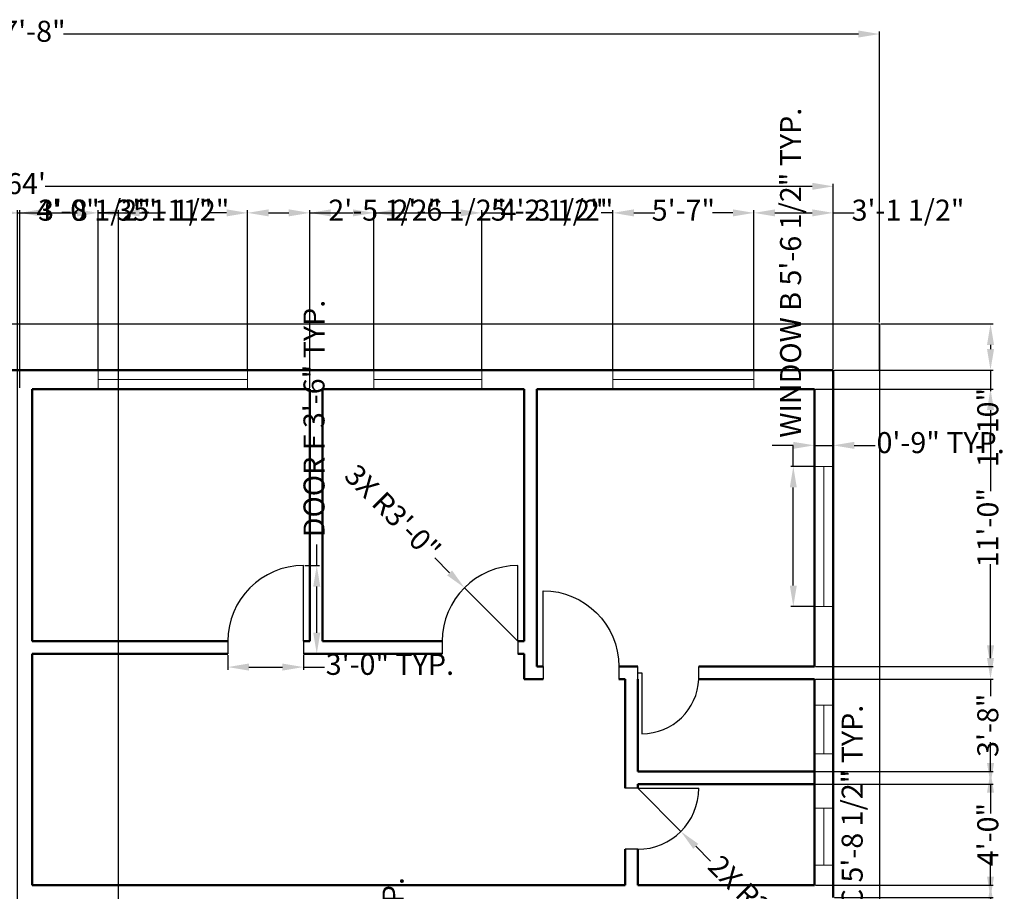
# Model space of a CAD drawing. Units: inches. Extents: x 3237 to 4201, y 2949 to 4053.
# Tile 5 of 5: x 3725 to 4193, y 3638 to 4053. Entities that reach past the tile are written whole.
import ezdxf

# ---------------------------------------------------------------- set-up
doc = ezdxf.new("R2010")
doc.units = ezdxf.units.IN
for name, color, linetype, lineweight in [('A-ANNO-DIMS', 2, 'Continuous', 18), ('A-DOOR', 3, 'Continuous', 25), ('A-GLAZ', 4, 'Continuous', 18), ('A-WALL', 7, 'Continuous', 50), ('C-PROP', 6, 'Continuous', 25)]:
    doc.layers.add(name, color=color, linetype=linetype, lineweight=lineweight)
doc.styles.get("Standard").update_dxf_attribs({"font": 'arial.ttf'})
doc.dimstyles.new('ISO-25', dxfattribs={"dimtxt": 10, "dimasz": 10, "dimexe": 1.25, "dimexo": 0.625, "dimtad": 0, "dimdec": 0, "dimlunit": 3, "dimtxsty": 'Standard', "dimcen": 2.5, "dimadec": 0, "dimazin": 0, "dimtfac": 1, "dimtdec": 0, "dimtmove": 0, "dimatfit": 3, "dimfxl": 1, "dimarcsym": 0})

# ---------------------------------------------------------------- blocks, each defined once
blk = doc.blocks.new('*D1')
at = {"layer": 'A-ANNO-DIMS', "color": 0, "lineweight": -2, "transparency": 16777216}
for p, q in [((3321.52, 3908.6), (3321.52, 4047.14)), ((4133.52, 3908.6), (4133.52, 4047.14)), ((3331.52, 4045.89), (3709.69, 4045.89)), ((4123.52, 4045.89), (3745.35, 4045.89))]:
    blk.add_line(p, q, dxfattribs=at)
at = {"layer": 'A-ANNO-DIMS', "color": 0, "transparency": 16777216}
for points in [[(3331.52, 4047.56), (3331.52, 4044.22), (3321.52, 4045.89)], [(4123.52, 4047.56), (4123.52, 4044.22), (4133.52, 4045.89)]]:
    blk.add_solid(points, dxfattribs=at)
at = {"layer": 'Defpoints', "color": 0, "transparency": 16777216}
for p in [(4133.52, 4045.89), (3321.52, 3907.98), (4133.52, 3907.98)]:
    blk.add_point(p, dxfattribs=at)
at = {"layer": 'A-ANNO-DIMS', "color": 0, "transparency": 16777216, "insert": (3727.52, 4045.89), "char_height": 10, "attachment_point": 5}
blk.add_mtext('67\'-8"', dxfattribs=at)
blk = doc.blocks.new('*D3')
at = {"layer": 'A-ANNO-DIMS', "color": 0, "lineweight": -2, "transparency": 16777216}
for p, q in [((3343.52, 3886.6), (3343.52, 3974.66)), ((3353.52, 3973.41), (3718.38, 3973.41)), ((4101.52, 3973.41), (3736.66, 3973.41)), ((4111.52, 3886.6), (4111.52, 3974.66))]:
    blk.add_line(p, q, dxfattribs=at)
at = {"layer": 'A-ANNO-DIMS', "color": 0, "transparency": 16777216}
for points in [[(3353.52, 3975.08), (3353.52, 3971.74), (3343.52, 3973.41)], [(4101.52, 3975.08), (4101.52, 3971.74), (4111.52, 3973.41)]]:
    blk.add_solid(points, dxfattribs=at)
at = {"layer": 'Defpoints', "color": 0, "transparency": 16777216}
for p in [(4111.52, 3973.41), (3343.52, 3885.98), (4111.52, 3885.98)]:
    blk.add_point(p, dxfattribs=at)
at = {"layer": 'A-ANNO-DIMS', "color": 0, "transparency": 16777216, "insert": (3727.52, 3973.41), "char_height": 10, "attachment_point": 5}
blk.add_mtext("64'", dxfattribs=at)
blk = doc.blocks.new('DOOR-29-OFFSET-A')
for p, q in [((0, 26), (0, 32)), ((0, 29), (2, 29)), ((2, 29), (2, 0)), ((29, 26), (29, 32))]:
    blk.add_line(p, q)
blk.add_arc((2, 27.02), 27.02, 270, 357.8382)
blk = doc.blocks.new('DOOR-36')
for p, q in [((36, 6), (36, 42)), ((0, 6), (0, 0)), ((36, 6), (36, 0))]:
    blk.add_line(p, q)
blk.add_arc((36, 6), 36, 90, 180)
blk = doc.blocks.new('DOOR-29')
for p, q in [((6, 29), (0, 29)), ((6, 29), (35, 29)), ((6, 0), (0, 0))]:
    blk.add_line(p, q)
blk.add_arc((6, 29), 29, 270, 0)
blk = doc.blocks.new('WIN-66p71IN')
for p, q in [((0, 66.71), (9, 66.71)), ((4.5, 0), (4.5, 66.71)), ((0, 0), (9, 0))]:
    blk.add_line(p, q)
blk = doc.blocks.new('*D23')
at = {"layer": 'A-ANNO-DIMS', "color": 0, "lineweight": -2, "transparency": 16777216}
for p, q in [((3903.41, 3494.25), (3903.41, 3504.25)), ((3898.15, 3494.25), (3904.66, 3494.25)), ((3903.41, 3464.98), (3903.41, 3484.25)), ((3898.15, 3454.98), (3904.66, 3454.98))]:
    blk.add_line(p, q, dxfattribs=at)
at = {"layer": 'A-ANNO-DIMS', "color": 0, "transparency": 16777216}
for points in [[(3901.75, 3484.25), (3905.08, 3484.25), (3903.41, 3494.25)], [(3901.75, 3464.98), (3905.08, 3464.98), (3903.41, 3454.98)]]:
    blk.add_solid(points, dxfattribs=at)
at = {"layer": 'Defpoints', "color": 0, "transparency": 16777216}
for p in [(3897.52, 3494.25), (3903.41, 3494.25), (3897.52, 3454.98)]:
    blk.add_point(p, dxfattribs=at)
at = {"layer": 'A-ANNO-DIMS', "color": 0, "transparency": 16777216, "insert": (3903.41, 3576.25), "char_height": 10, "attachment_point": 5, "rotation": 90}
blk.add_mtext('DOOR E 3\'-3 1/2" TYP.', dxfattribs=at)
blk = doc.blocks.new('*D25')
at = {"layer": 'A-ANNO-DIMS', "color": 0, "lineweight": -2, "transparency": 16777216}
for p, q in [((3865.82, 3792.98), (3865.82, 3802.98)), ((3860.15, 3792.98), (3867.07, 3792.98)), ((3865.82, 3760.98), (3865.82, 3782.98)), ((3860.15, 3750.98), (3867.07, 3750.98))]:
    blk.add_line(p, q, dxfattribs=at)
at = {"layer": 'A-ANNO-DIMS', "color": 0, "transparency": 16777216}
for points in [[(3864.16, 3782.98), (3867.49, 3782.98), (3865.82, 3792.98)], [(3864.16, 3760.98), (3867.49, 3760.98), (3865.82, 3750.98)]]:
    blk.add_solid(points, dxfattribs=at)
at = {"layer": 'Defpoints', "color": 0, "transparency": 16777216}
for p in [(3859.52, 3792.98), (3865.82, 3792.98), (3859.52, 3750.98)]:
    blk.add_point(p, dxfattribs=at)
at = {"layer": 'A-ANNO-DIMS', "color": 0, "transparency": 16777216, "insert": (3865.82, 3862.94), "char_height": 10, "attachment_point": 5, "rotation": 90}
blk.add_mtext('DOOR F 3\'-6" TYP.', dxfattribs=at)
blk = doc.blocks.new('*D26')
at = {"layer": 'A-ANNO-DIMS', "color": 0, "lineweight": -2, "transparency": 16777216}
for p, q in [((3823.52, 3750.35), (3823.52, 3743.43)), ((3859.52, 3750.35), (3859.52, 3743.43)), ((3833.52, 3744.68), (3849.52, 3744.68)), ((3859.52, 3744.68), (3869.52, 3744.68))]:
    blk.add_line(p, q, dxfattribs=at)
at = {"layer": 'A-ANNO-DIMS', "color": 0, "transparency": 16777216}
for points in [[(3833.52, 3746.35), (3833.52, 3743.01), (3823.52, 3744.68)], [(3849.52, 3746.35), (3849.52, 3743.01), (3859.52, 3744.68)]]:
    blk.add_solid(points, dxfattribs=at)
at = {"layer": 'Defpoints', "color": 0, "transparency": 16777216}
for p in [(3823.52, 3750.98), (3859.52, 3750.98), (3859.52, 3744.68)]:
    blk.add_point(p, dxfattribs=at)
at = {"layer": 'A-ANNO-DIMS', "color": 0, "transparency": 16777216, "insert": (3900.62, 3744.68), "char_height": 10, "attachment_point": 5}
blk.add_mtext('3\'-0" TYP.', dxfattribs=at)
blk = doc.blocks.new('*D29')
at = {"layer": 'A-ANNO-DIMS', "color": 0, "lineweight": -2, "transparency": 16777216}
for p, q in [((4092.52, 3840.16), (4092.52, 3850.16)), ((4101.9, 3840.16), (4091.27, 3840.16)), ((4092.52, 3783.45), (4092.52, 3830.16)), ((4101.9, 3773.45), (4091.27, 3773.45))]:
    blk.add_line(p, q, dxfattribs=at)
at = {"layer": 'A-ANNO-DIMS', "color": 0, "transparency": 16777216}
for points in [[(4090.85, 3830.16), (4094.18, 3830.16), (4092.52, 3840.16)], [(4090.85, 3783.45), (4094.18, 3783.45), (4092.52, 3773.45)]]:
    blk.add_solid(points, dxfattribs=at)
at = {"layer": 'Defpoints', "color": 0, "transparency": 16777216}
for p in [(4092.52, 3840.16), (4102.52, 3840.16), (4102.52, 3773.45)]:
    blk.add_point(p, dxfattribs=at)
at = {"layer": 'A-ANNO-DIMS', "color": 0, "transparency": 16777216, "insert": (4092.52, 3932.31), "char_height": 10, "attachment_point": 5, "rotation": 90}
blk.add_mtext('WINDOW B 5\'-6 1/2" TYP.', dxfattribs=at)
blk = doc.blocks.new('*D30')
at = {"layer": 'A-ANNO-DIMS', "color": 0, "lineweight": -2, "transparency": 16777216}
for p, q in [((4092.52, 3850.17), (4082.52, 3850.17)), ((4102.52, 3840.78), (4102.52, 3851.42)), ((4102.52, 3850.17), (4111.52, 3850.17)), ((4111.52, 3840.78), (4111.52, 3851.42)), ((4121.52, 3850.17), (4131.52, 3850.17))]:
    blk.add_line(p, q, dxfattribs=at)
at = {"layer": 'A-ANNO-DIMS', "color": 0, "transparency": 16777216}
for points in [[(4092.52, 3851.83), (4092.52, 3848.5), (4102.52, 3850.17)], [(4121.52, 3851.83), (4121.52, 3848.5), (4111.52, 3850.17)]]:
    blk.add_solid(points, dxfattribs=at)
at = {"layer": 'Defpoints', "color": 0, "transparency": 16777216}
for p in [(4111.52, 3850.17), (4102.52, 3840.16), (4111.52, 3840.16)]:
    blk.add_point(p, dxfattribs=at)
at = {"layer": 'A-ANNO-DIMS', "color": 0, "transparency": 16777216, "insert": (4162.62, 3850.17), "char_height": 10, "attachment_point": 5}
blk.add_mtext('0\'-9" TYP.', dxfattribs=at)
blk = doc.blocks.new('*D31')
at = {"layer": 'A-ANNO-DIMS', "color": 0, "lineweight": -2, "transparency": 16777216}
for p, q in [((4121.81, 3555.85), (4121.81, 3565.85)), ((4112.15, 3555.85), (4123.06, 3555.85)), ((4121.81, 3497.24), (4121.81, 3545.85)), ((4112.15, 3487.24), (4123.06, 3487.24))]:
    blk.add_line(p, q, dxfattribs=at)
at = {"layer": 'A-ANNO-DIMS', "color": 0, "transparency": 16777216}
for points in [[(4120.15, 3545.85), (4123.48, 3545.85), (4121.81, 3555.85)], [(4120.15, 3497.24), (4123.48, 3497.24), (4121.81, 3487.24)]]:
    blk.add_solid(points, dxfattribs=at)
at = {"layer": 'Defpoints', "color": 0, "transparency": 16777216}
for p in [(4111.52, 3555.85), (4121.81, 3555.85), (4111.52, 3487.24)]:
    blk.add_point(p, dxfattribs=at)
at = {"layer": 'A-ANNO-DIMS', "color": 0, "transparency": 16777216, "insert": (4121.81, 3648.38), "char_height": 10, "attachment_point": 5, "rotation": 90}
blk.add_mtext('WINDOW C 5\'-8 1/2" TYP.', dxfattribs=at)
blk = doc.blocks.new('*D42')
at = {"layer": 'A-ANNO-DIMS', "color": 0, "lineweight": -2, "transparency": 16777216}
for p, q in [((3680.25, 3886.6), (3680.25, 3962.03)), ((3690.25, 3960.78), (3714.52, 3960.78)), ((3724.52, 3877.6), (3724.52, 3962.03)), ((3724.52, 3960.78), (3734.52, 3960.78))]:
    blk.add_line(p, q, dxfattribs=at)
at = {"layer": 'A-ANNO-DIMS', "color": 0, "transparency": 16777216}
for points in [[(3690.25, 3962.45), (3690.25, 3959.11), (3680.25, 3960.78)], [(3714.52, 3962.45), (3714.52, 3959.11), (3724.52, 3960.78)]]:
    blk.add_solid(points, dxfattribs=at)
at = {"layer": 'Defpoints', "color": 0, "transparency": 16777216}
for p in [(3724.52, 3960.78), (3680.25, 3885.98), (3724.52, 3876.98)]:
    blk.add_point(p, dxfattribs=at)
at = {"layer": 'A-ANNO-DIMS', "color": 0, "transparency": 16777216, "insert": (3760.09, 3960.78), "char_height": 10, "attachment_point": 5}
blk.add_mtext('3\'-8 1/2"', dxfattribs=at)
blk = doc.blocks.new('*D43')
at = {"layer": 'A-ANNO-DIMS', "color": 0, "lineweight": -2, "transparency": 16777216}
for p, q in [((3724.52, 3877.6), (3724.52, 3962.03)), ((3734.52, 3960.78), (3751.85, 3960.78)), ((3761.85, 3886.6), (3761.85, 3962.03)), ((3761.85, 3960.78), (3771.85, 3960.78))]:
    blk.add_line(p, q, dxfattribs=at)
at = {"layer": 'A-ANNO-DIMS', "color": 0, "transparency": 16777216}
for points in [[(3734.52, 3962.45), (3734.52, 3959.11), (3724.52, 3960.78)], [(3751.85, 3962.45), (3751.85, 3959.11), (3761.85, 3960.78)]]:
    blk.add_solid(points, dxfattribs=at)
at = {"layer": 'Defpoints', "color": 0, "transparency": 16777216}
for p in [(3761.85, 3960.78), (3761.85, 3885.98), (3724.52, 3876.98)]:
    blk.add_point(p, dxfattribs=at)
at = {"layer": 'A-ANNO-DIMS', "color": 0, "transparency": 16777216, "insert": (3797.42, 3960.78), "char_height": 10, "attachment_point": 5}
blk.add_mtext('3\'-1 1/2"', dxfattribs=at)
blk = doc.blocks.new('*D44')
at = {"layer": 'A-ANNO-DIMS', "color": 0, "lineweight": -2, "transparency": 16777216}
for p, q in [((3761.85, 3886.6), (3761.85, 3962.03)), ((3771.85, 3960.78), (3779.58, 3960.78)), ((3822.9, 3960.78), (3815.18, 3960.78)), ((3832.9, 3886.6), (3832.9, 3962.03))]:
    blk.add_line(p, q, dxfattribs=at)
at = {"layer": 'A-ANNO-DIMS', "color": 0, "transparency": 16777216}
for points in [[(3771.85, 3962.45), (3771.85, 3959.11), (3761.85, 3960.78)], [(3822.9, 3962.45), (3822.9, 3959.11), (3832.9, 3960.78)]]:
    blk.add_solid(points, dxfattribs=at)
at = {"layer": 'Defpoints', "color": 0, "transparency": 16777216}
for p in [(3832.9, 3960.78), (3761.85, 3885.98), (3832.9, 3885.98)]:
    blk.add_point(p, dxfattribs=at)
at = {"layer": 'A-ANNO-DIMS', "color": 0, "transparency": 16777216, "insert": (3797.38, 3960.78), "char_height": 10, "attachment_point": 5}
blk.add_mtext('5\'-11"', dxfattribs=at)
blk = doc.blocks.new('*D45')
at = {"layer": 'A-ANNO-DIMS', "color": 0, "lineweight": -2, "transparency": 16777216}
for p, q in [((3832.9, 3886.6), (3832.9, 3962.03)), ((3842.9, 3960.78), (3852.52, 3960.78)), ((3862.52, 3877.6), (3862.52, 3962.03)), ((3862.52, 3960.78), (3872.52, 3960.78))]:
    blk.add_line(p, q, dxfattribs=at)
at = {"layer": 'A-ANNO-DIMS', "color": 0, "transparency": 16777216}
for points in [[(3842.9, 3962.45), (3842.9, 3959.11), (3832.9, 3960.78)], [(3852.52, 3962.45), (3852.52, 3959.11), (3862.52, 3960.78)]]:
    blk.add_solid(points, dxfattribs=at)
at = {"layer": 'Defpoints', "color": 0, "transparency": 16777216}
for p in [(3862.52, 3960.78), (3832.9, 3885.98), (3862.52, 3876.98)]:
    blk.add_point(p, dxfattribs=at)
at = {"layer": 'A-ANNO-DIMS', "color": 0, "transparency": 16777216, "insert": (3898.17, 3960.78), "char_height": 10, "attachment_point": 5}
blk.add_mtext('2\'-5 1/2"', dxfattribs=at)
blk = doc.blocks.new('*D46')
at = {"layer": 'A-ANNO-DIMS', "color": 0, "lineweight": -2, "transparency": 16777216}
for p, q in [((3862.52, 3877.6), (3862.52, 3962.03)), ((3872.52, 3960.78), (3883.05, 3960.78)), ((3893.05, 3886.6), (3893.05, 3962.03)), ((3893.05, 3960.78), (3903.05, 3960.78))]:
    blk.add_line(p, q, dxfattribs=at)
at = {"layer": 'A-ANNO-DIMS', "color": 0, "transparency": 16777216}
for points in [[(3872.52, 3962.45), (3872.52, 3959.11), (3862.52, 3960.78)], [(3883.05, 3962.45), (3883.05, 3959.11), (3893.05, 3960.78)]]:
    blk.add_solid(points, dxfattribs=at)
at = {"layer": 'Defpoints', "color": 0, "transparency": 16777216}
for p in [(3893.05, 3960.78), (3893.05, 3885.98), (3862.52, 3876.98)]:
    blk.add_point(p, dxfattribs=at)
at = {"layer": 'A-ANNO-DIMS', "color": 0, "transparency": 16777216, "insert": (3928.7, 3960.78), "char_height": 10, "attachment_point": 5}
blk.add_mtext('2\'-6 1/2"', dxfattribs=at)
blk = doc.blocks.new('*D47')
at = {"layer": 'A-ANNO-DIMS', "color": 0, "lineweight": -2, "transparency": 16777216}
for p, q in [((3893.05, 3886.6), (3893.05, 3962.03)), ((3903.05, 3960.78), (3934.32, 3960.78)), ((3944.32, 3886.6), (3944.32, 3962.03)), ((3944.32, 3960.78), (3954.32, 3960.78))]:
    blk.add_line(p, q, dxfattribs=at)
at = {"layer": 'A-ANNO-DIMS', "color": 0, "transparency": 16777216}
for points in [[(3903.05, 3962.45), (3903.05, 3959.11), (3893.05, 3960.78)], [(3934.32, 3962.45), (3934.32, 3959.11), (3944.32, 3960.78)]]:
    blk.add_solid(points, dxfattribs=at)
at = {"layer": 'Defpoints', "color": 0, "transparency": 16777216}
for p in [(3944.32, 3960.78), (3893.05, 3885.98), (3944.32, 3885.98)]:
    blk.add_point(p, dxfattribs=at)
at = {"layer": 'A-ANNO-DIMS', "color": 0, "transparency": 16777216, "insert": (3980.09, 3960.78), "char_height": 10, "attachment_point": 5}
blk.add_mtext('4\'-3 1/2"', dxfattribs=at)
blk = doc.blocks.new('*D48')
at = {"layer": 'A-ANNO-DIMS', "color": 0, "lineweight": -2, "transparency": 16777216}
for p, q in [((3934.32, 3960.78), (3924.32, 3960.78)), ((3944.32, 3886.6), (3944.32, 3962.03)), ((3944.32, 3960.78), (3949.92, 3960.78)), ((4006.66, 3960.78), (4001.06, 3960.78)), ((4006.66, 3886.6), (4006.66, 3962.03)), ((4016.66, 3960.78), (4026.66, 3960.78))]:
    blk.add_line(p, q, dxfattribs=at)
at = {"layer": 'A-ANNO-DIMS', "color": 0, "transparency": 16777216}
for points in [[(3934.32, 3962.45), (3934.32, 3959.11), (3944.32, 3960.78)], [(4016.66, 3962.45), (4016.66, 3959.11), (4006.66, 3960.78)]]:
    blk.add_solid(points, dxfattribs=at)
at = {"layer": 'Defpoints', "color": 0, "transparency": 16777216}
for p in [(4006.66, 3960.78), (3944.32, 3885.98), (4006.66, 3885.98)]:
    blk.add_point(p, dxfattribs=at)
at = {"layer": 'A-ANNO-DIMS', "color": 0, "transparency": 16777216, "insert": (3975.49, 3960.78), "char_height": 10, "attachment_point": 5}
blk.add_mtext('5\'-2 1/2"', dxfattribs=at)
blk = doc.blocks.new('*D49')
at = {"layer": 'A-ANNO-DIMS', "color": 0, "lineweight": -2, "transparency": 16777216}
for p, q in [((4006.66, 3886.6), (4006.66, 3962.03)), ((4016.66, 3960.78), (4026.31, 3960.78)), ((4063.8, 3960.78), (4054.14, 3960.78)), ((4073.8, 3886.6), (4073.8, 3962.03))]:
    blk.add_line(p, q, dxfattribs=at)
at = {"layer": 'A-ANNO-DIMS', "color": 0, "transparency": 16777216}
for points in [[(4016.66, 3962.45), (4016.66, 3959.11), (4006.66, 3960.78)], [(4063.8, 3962.45), (4063.8, 3959.11), (4073.8, 3960.78)]]:
    blk.add_solid(points, dxfattribs=at)
at = {"layer": 'Defpoints', "color": 0, "transparency": 16777216}
for p in [(4073.8, 3960.78), (4006.66, 3885.98), (4073.8, 3885.98)]:
    blk.add_point(p, dxfattribs=at)
at = {"layer": 'A-ANNO-DIMS', "color": 0, "transparency": 16777216, "insert": (4040.23, 3960.78), "char_height": 10, "attachment_point": 5}
blk.add_mtext('5\'-7"', dxfattribs=at)
blk = doc.blocks.new('*D50')
at = {"layer": 'A-ANNO-DIMS', "color": 0, "lineweight": -2, "transparency": 16777216}
for p, q in [((4073.8, 3886.6), (4073.8, 3962.03)), ((4083.8, 3960.78), (4101.52, 3960.78)), ((4111.52, 3886.6), (4111.52, 3962.03)), ((4111.52, 3960.78), (4121.52, 3960.78))]:
    blk.add_line(p, q, dxfattribs=at)
at = {"layer": 'A-ANNO-DIMS', "color": 0, "transparency": 16777216}
for points in [[(4083.8, 3962.45), (4083.8, 3959.11), (4073.8, 3960.78)], [(4101.52, 3962.45), (4101.52, 3959.11), (4111.52, 3960.78)]]:
    blk.add_solid(points, dxfattribs=at)
at = {"layer": 'Defpoints', "color": 0, "transparency": 16777216}
for p in [(4111.52, 3960.78), (4073.8, 3885.98), (4111.52, 3885.98)]:
    blk.add_point(p, dxfattribs=at)
at = {"layer": 'A-ANNO-DIMS', "color": 0, "transparency": 16777216, "insert": (4147.09, 3960.78), "char_height": 10, "attachment_point": 5}
blk.add_mtext('3\'-1 1/2"', dxfattribs=at)
blk = doc.blocks.new('*D52')
at = {"layer": 'A-ANNO-DIMS', "color": 0, "lineweight": -2, "transparency": 16777216}
for p, q in [((4134.15, 3907.98), (4187.57, 3907.98)), ((4186.32, 3897.98), (4186.32, 3895.98)), ((4112.15, 3885.98), (4187.57, 3885.98)), ((4186.32, 3885.98), (4186.32, 3875.98))]:
    blk.add_line(p, q, dxfattribs=at)
at = {"layer": 'A-ANNO-DIMS', "color": 0, "transparency": 16777216}
for points in [[(4184.66, 3897.98), (4187.99, 3897.98), (4186.32, 3907.98)], [(4184.66, 3895.98), (4187.99, 3895.98), (4186.32, 3885.98)]]:
    blk.add_solid(points, dxfattribs=at)
at = {"layer": 'Defpoints', "color": 0, "transparency": 16777216}
for p in [(4133.52, 3907.98), (4111.52, 3885.98), (4186.32, 3885.98)]:
    blk.add_point(p, dxfattribs=at)
at = {"layer": 'A-ANNO-DIMS', "color": 0, "transparency": 16777216, "insert": (4186.32, 3858.65), "char_height": 10, "attachment_point": 5, "rotation": 90}
blk.add_mtext('1\'-10"', dxfattribs=at)
blk = doc.blocks.new('*D65')
at = {"layer": 'A-ANNO-DIMS', "color": 0, "lineweight": -2, "transparency": 16777216}
for p, q in [((4186.32, 3644.98), (4186.32, 3654.98)), ((4112.15, 3634.98), (4187.57, 3634.98)), ((4186.32, 3634.98), (4186.32, 3630.89)), ((4186.32, 3598.98), (4186.32, 3603.07)), ((4112.15, 3598.98), (4187.57, 3598.98)), ((4186.32, 3588.98), (4186.32, 3578.98))]:
    blk.add_line(p, q, dxfattribs=at)
at = {"layer": 'A-ANNO-DIMS', "color": 0, "transparency": 16777216}
for points in [[(4184.66, 3644.98), (4187.99, 3644.98), (4186.32, 3634.98)], [(4184.66, 3588.98), (4187.99, 3588.98), (4186.32, 3598.98)]]:
    blk.add_solid(points, dxfattribs=at)
at = {"layer": 'Defpoints', "color": 0, "transparency": 16777216}
for p in [(4111.52, 3634.98), (4186.32, 3634.98), (4111.52, 3598.98)]:
    blk.add_point(p, dxfattribs=at)
at = {"layer": 'A-ANNO-DIMS', "color": 0, "transparency": 16777216, "insert": (4186.32, 3616.98), "char_height": 10, "attachment_point": 5, "rotation": 90}
blk.add_mtext('3\'-0"', dxfattribs=at)
blk = doc.blocks.new('*D66')
at = {"layer": 'A-ANNO-DIMS', "color": 0, "lineweight": -2, "transparency": 16777216}
for p, q in [((4186.32, 3698.98), (4186.32, 3708.98)), ((4103.15, 3688.98), (4187.57, 3688.98)), ((4186.32, 3688.98), (4186.32, 3679.1)), ((4186.32, 3640.98), (4186.32, 3650.86)), ((4103.15, 3640.98), (4187.57, 3640.98)), ((4186.32, 3630.98), (4186.32, 3620.98))]:
    blk.add_line(p, q, dxfattribs=at)
at = {"layer": 'A-ANNO-DIMS', "color": 0, "transparency": 16777216}
for points in [[(4184.66, 3698.98), (4187.99, 3698.98), (4186.32, 3688.98)], [(4184.66, 3630.98), (4187.99, 3630.98), (4186.32, 3640.98)]]:
    blk.add_solid(points, dxfattribs=at)
at = {"layer": 'Defpoints', "color": 0, "transparency": 16777216}
for p in [(4102.52, 3688.98), (4186.32, 3688.98), (4102.52, 3640.98)]:
    blk.add_point(p, dxfattribs=at)
at = {"layer": 'A-ANNO-DIMS', "color": 0, "transparency": 16777216, "insert": (4186.32, 3664.98), "char_height": 10, "attachment_point": 5, "rotation": 90}
blk.add_mtext('4\'-0"', dxfattribs=at)
blk = doc.blocks.new('*D67')
at = {"layer": 'A-ANNO-DIMS', "color": 0, "lineweight": -2, "transparency": 16777216}
for p, q in [((4186.32, 3748.98), (4186.32, 3758.98)), ((4103.15, 3738.98), (4187.57, 3738.98)), ((4186.32, 3738.98), (4186.32, 3730.89)), ((4186.32, 3694.98), (4186.32, 3703.07)), ((4103.15, 3694.98), (4187.57, 3694.98)), ((4186.32, 3684.98), (4186.32, 3674.98))]:
    blk.add_line(p, q, dxfattribs=at)
at = {"layer": 'A-ANNO-DIMS', "color": 0, "transparency": 16777216}
for points in [[(4184.66, 3748.98), (4187.99, 3748.98), (4186.32, 3738.98)], [(4184.66, 3684.98), (4187.99, 3684.98), (4186.32, 3694.98)]]:
    blk.add_solid(points, dxfattribs=at)
at = {"layer": 'Defpoints', "color": 0, "transparency": 16777216}
for p in [(4102.52, 3738.98), (4186.32, 3738.98), (4102.52, 3694.98)]:
    blk.add_point(p, dxfattribs=at)
at = {"layer": 'A-ANNO-DIMS', "color": 0, "transparency": 16777216, "insert": (4186.32, 3716.98), "char_height": 10, "attachment_point": 5, "rotation": 90}
blk.add_mtext('3\'-8"', dxfattribs=at)
blk = doc.blocks.new('*D68')
at = {"layer": 'A-ANNO-DIMS', "color": 0, "lineweight": -2, "transparency": 16777216}
for p, q in [((4103.15, 3876.98), (4187.57, 3876.98)), ((4186.32, 3866.98), (4186.32, 3828.31)), ((4186.32, 3754.98), (4186.32, 3793.65)), ((4103.15, 3744.98), (4187.57, 3744.98))]:
    blk.add_line(p, q, dxfattribs=at)
at = {"layer": 'A-ANNO-DIMS', "color": 0, "transparency": 16777216}
for points in [[(4184.66, 3866.98), (4187.99, 3866.98), (4186.32, 3876.98)], [(4184.66, 3754.98), (4187.99, 3754.98), (4186.32, 3744.98)]]:
    blk.add_solid(points, dxfattribs=at)
at = {"layer": 'Defpoints', "color": 0, "transparency": 16777216}
for p in [(4102.52, 3876.98), (4186.32, 3876.98), (4102.52, 3744.98)]:
    blk.add_point(p, dxfattribs=at)
at = {"layer": 'A-ANNO-DIMS', "color": 0, "transparency": 16777216, "insert": (4186.32, 3810.98), "char_height": 10, "attachment_point": 5, "rotation": 90}
blk.add_mtext('11\'-0"', dxfattribs=at)
blk = doc.blocks.new('*D83')
at = {"layer": 'A-ANNO-DIMS', "color": 0, "lineweight": -2, "transparency": 16777216}
for p, q in [((3713.52, 3960.78), (3703.52, 3960.78)), ((3723.52, 3193.4), (3723.52, 3962.03)), ((3723.52, 3960.78), (3733.4, 3960.78)), ((3771.52, 3960.78), (3761.64, 3960.78)), ((3771.52, 3193.4), (3771.52, 3962.03)), ((3781.52, 3960.78), (3791.52, 3960.78))]:
    blk.add_line(p, q, dxfattribs=at)
at = {"layer": 'A-ANNO-DIMS', "color": 0, "transparency": 16777216}
for points in [[(3713.52, 3962.45), (3713.52, 3959.11), (3723.52, 3960.78)], [(3781.52, 3962.45), (3781.52, 3959.11), (3771.52, 3960.78)]]:
    blk.add_solid(points, dxfattribs=at)
at = {"layer": 'Defpoints', "color": 0, "transparency": 16777216}
for p in [(3771.52, 3960.78), (3723.52, 3192.78), (3771.52, 3192.78)]:
    blk.add_point(p, dxfattribs=at)
at = {"layer": 'A-ANNO-DIMS', "color": 0, "transparency": 16777216, "insert": (3747.52, 3960.78), "char_height": 10, "attachment_point": 5}
blk.add_mtext('4\'-0"', dxfattribs=at)
blk = doc.blocks.new('*D92')
at = {"layer": 'A-ANNO-DIMS', "color": 0, "lineweight": -2, "transparency": 16777216}
for p, q in [((3921.92, 3796.58), (3928.99, 3789.51)), ((3961.52, 3756.98), (3936.07, 3782.44))]:
    blk.add_line(p, q, dxfattribs=at)
at = {"layer": 'A-ANNO-DIMS', "color": 0, "transparency": 16777216}
blk.add_solid([(3930.17, 3790.68), (3927.82, 3788.33), (3936.07, 3782.44)], dxfattribs=at)
at = {"layer": 'Defpoints', "color": 0, "transparency": 16777216}
for p in [(3936.07, 3782.44), (3961.52, 3756.98)]:
    blk.add_point(p, dxfattribs=at)
at = {"layer": 'A-ANNO-DIMS', "color": 0, "transparency": 16777216, "insert": (3901.11, 3817.4), "char_height": 10, "attachment_point": 5, "rotation": 315.0004}
blk.add_mtext('3X R3\'-0"', dxfattribs=at)
blk = doc.blocks.new('*D93')
at = {"layer": 'A-ANNO-DIMS', "color": 0, "lineweight": -2, "transparency": 16777216}
for p, q in [((4018.52, 3686.98), (4039.03, 3666.47)), ((4053.17, 3652.33), (4046.1, 3659.4))]:
    blk.add_line(p, q, dxfattribs=at)
at = {"layer": 'A-ANNO-DIMS', "color": 0, "transparency": 16777216}
blk.add_solid([(4047.28, 3660.58), (4044.92, 3658.22), (4039.03, 3666.47)], dxfattribs=at)
at = {"layer": 'Defpoints', "color": 0, "transparency": 16777216}
for p in [(4018.52, 3686.98), (4039.03, 3666.47)]:
    blk.add_point(p, dxfattribs=at)
at = {"layer": 'A-ANNO-DIMS', "color": 0, "transparency": 16777216, "insert": (4074.05, 3631.45), "char_height": 10, "attachment_point": 5, "rotation": 314.9995}
blk.add_mtext('2X R2\'-5"', dxfattribs=at)

msp = doc.modelspace()

# ---------------------------------------------------------------- linework, layer by layer
at = {"layer": 'A-GLAZ'}
for p, q in [((3761.85, 3876.98), (3761.85, 3885.98)), ((3832.9, 3876.98), (3832.9, 3885.98)), ((3893.05, 3876.98), (3893.05, 3885.98)), ((3944.32, 3876.98), (3944.32, 3885.98)), ((4006.66, 3876.98), (4006.66, 3885.98)), ((4073.8, 3876.98), (4073.8, 3885.98)), ((3832.9, 3881.48), (3761.85, 3881.48)), ((3944.32, 3881.48), (3893.05, 3881.48)), ((4073.8, 3881.48), (4006.66, 3881.48)), ((4102.52, 3726.49), (4111.52, 3726.49)), ((4107.02, 3726.49), (4107.02, 3703.36)), ((4102.52, 3703.36), (4111.52, 3703.36)), ((4102.52, 3677.47), (4111.52, 3677.47)), ((4107.02, 3650.37), (4107.02, 3677.47)), ((4102.52, 3650.37), (4111.52, 3650.37))]:
    msp.add_line(p, q, dxfattribs=at)
at = {"layer": 'A-WALL'}
for p, q in [((4111.52, 3885.98), (3343.52, 3885.98)), ((4111.52, 3634.98), (4111.52, 3885.98)), ((3730.52, 3876.98), (3730.52, 3756.98)), ((3862.52, 3876.98), (3730.52, 3876.98)), ((3862.52, 3756.98), (3862.52, 3876.98)), ((3868.52, 3756.98), (3868.52, 3876.98)), ((3964.52, 3876.98), (3868.52, 3876.98)), ((3964.52, 3756.98), (3964.52, 3876.98)), ((4102.52, 3876.98), (3970.52, 3876.98)), ((3970.52, 3744.98), (3970.52, 3876.98)), ((4102.52, 3744.98), (4102.52, 3876.98)), ((3823.52, 3756.98), (3730.52, 3756.98)), ((3862.52, 3756.98), (3859.52, 3756.98)), ((3925.52, 3756.98), (3868.52, 3756.98)), ((3964.52, 3756.98), (3961.52, 3756.98)), ((3730.52, 3750.98), (3730.52, 3640.98)), ((3823.52, 3750.98), (3730.52, 3750.98)), ((3925.52, 3750.98), (3859.52, 3750.98)), ((3964.52, 3750.98), (3961.52, 3750.98)), ((3964.52, 3738.98), (3964.52, 3750.98)), ((3973.52, 3744.98), (3970.52, 3744.98)), ((4018.52, 3744.98), (4009.52, 3744.98)), ((4102.52, 3744.98), (4047.52, 3744.98)), ((3973.52, 3738.98), (3964.52, 3738.98)), ((4012.52, 3738.98), (4009.52, 3738.98)), ((4012.52, 3686.98), (4012.52, 3738.98)), ((4018.52, 3694.98), (4018.52, 3738.98)), ((4102.52, 3738.98), (4047.52, 3738.98)), ((4102.52, 3640.98), (4102.52, 3738.98)), ((4102.52, 3694.98), (4018.52, 3694.98)), ((4102.52, 3688.98), (4018.52, 3688.98)), ((4018.52, 3686.98), (4018.52, 3688.98)), ((4012.52, 3640.98), (4012.52, 3657.98)), ((4018.52, 3640.98), (4018.52, 3657.98)), ((3970.52, 3640.98), (3730.52, 3640.98)), ((4012.52, 3640.98), (3964.52, 3640.98)), ((4102.52, 3640.98), (4018.52, 3640.98))]:
    msp.add_line(p, q, dxfattribs=at)
at = {"layer": 'C-PROP'}
for p, q in [((3321.52, 3907.98), (4133.52, 3907.98)), ((4133.52, 3885.98), (4133.52, 3907.98)), ((4133.52, 3907.98), (4133.52, 3007.98))]:
    msp.add_line(p, q, dxfattribs=at)

# ---------------------------------------------------------------- block references
at = {"layer": 'A-DOOR'}
for name, p in [('DOOR-36', (3823.52, 3750.98)), ('DOOR-36', (3925.52, 3750.98)), ('DOOR-29-OFFSET-A', (4018.52, 3712.98)), ('DOOR-29', (4012.52, 3657.98))]:
    msp.add_blockref(name, p, dxfattribs=at)
at = {"layer": 'A-DOOR', "extrusion": (0, 0, -1), "zscale": -1}
msp.add_blockref('DOOR-36', (-4009.52, 3738.98), dxfattribs=at)
at = {"layer": 'A-GLAZ'}
msp.add_blockref('WIN-66p71IN', (4102.52, 3773.45), dxfattribs=at)

# ---------------------------------------------------------------- dimensions: what is measured, and where the dimension line sits
at = {"layer": 'A-ANNO-DIMS'}
for base, p1, p2, override, picture, middle in [((4133.52, 4045.89), (3321.52, 3907.98), (4133.52, 3907.98), {"dimclrd": 0, "dimclre": 0, "dimclrt": 0}, '*D1', (3727.52, 4045.89)), ((4111.52, 3973.41), (3343.52, 3885.98), (4111.52, 3885.98), {"dimclrd": 0, "dimclre": 0, "dimclrt": 0}, '*D3', (3727.52, 3973.41)), ((3724.52, 3960.78), (3680.25, 3885.98), (3724.52, 3876.98), {"dimdec": 1, "dimlfac": 1, "dimrnd": 0, "dimzin": 1, "dimdsep": 46, "dimlunit": 4, "dimfrac": 2}, '*D42', (3760.09, 3960.78)), ((3761.85, 3960.78), (3724.52, 3876.98), (3761.85, 3885.98), {"dimdec": 1, "dimlfac": 1, "dimrnd": 0, "dimzin": 1, "dimdsep": 46, "dimlunit": 4, "dimfrac": 2}, '*D43', (3797.42, 3960.78)), ((3862.52, 3960.78), (3832.9, 3885.98), (3862.52, 3876.98), {"dimdec": 1, "dimlfac": 1, "dimrnd": 0, "dimzin": 1, "dimdsep": 46, "dimlunit": 4, "dimfrac": 2}, '*D45', (3898.17, 3960.78)), ((3893.05, 3960.78), (3862.52, 3876.98), (3893.05, 3885.98), {"dimdec": 1, "dimlfac": 1, "dimrnd": 0, "dimzin": 1, "dimdsep": 46, "dimlunit": 4, "dimfrac": 2}, '*D46', (3928.7, 3960.78)), ((3944.32, 3960.78), (3893.05, 3885.98), (3944.32, 3885.98), {"dimdec": 1, "dimlfac": 1, "dimrnd": 0, "dimzin": 1, "dimdsep": 46, "dimlunit": 4, "dimfrac": 2}, '*D47', (3980.09, 3960.78)), ((4006.66, 3960.78), (3944.32, 3885.98), (4006.66, 3885.98), {"dimdec": 1, "dimlfac": 1, "dimrnd": 0, "dimzin": 1, "dimdsep": 46, "dimlunit": 4, "dimfrac": 2}, '*D48', (3975.49, 3960.78)), ((4111.52, 3960.78), (4073.8, 3885.98), (4111.52, 3885.98), {"dimdec": 1, "dimlfac": 1, "dimrnd": 0, "dimzin": 1, "dimdsep": 46, "dimlunit": 4, "dimfrac": 2}, '*D50', (4147.09, 3960.78)), ((3771.52, 3960.78), (3723.52, 3192.78), (3771.52, 3192.78), {"dimdec": 1, "dimlfac": 1, "dimrnd": 0, "dimzin": 1, "dimdsep": 46, "dimlunit": 4, "dimfrac": 2}, '*D83', (3747.52, 3960.78)), ((3832.9, 3960.7796), (3761.8525, 3885.9796), (3832.9, 3885.9796), {"dimdec": 1, "dimlfac": 1, "dimrnd": 0, "dimzin": 1, "dimdsep": 46, "dimlunit": 4, "dimfrac": 2}, '*D44', (3797.3762, 3960.7796)), ((4073.8, 3960.78), (4006.66, 3885.98), (4073.8, 3885.98), {"dimdec": 1, "dimlfac": 1, "dimrnd": 0, "dimzin": 1, "dimdsep": 46, "dimlunit": 4, "dimfrac": 2}, '*D49', (4040.23, 3960.78))]:
    dim = msp.add_linear_dim(base=base, p1=p1, p2=p2, dimstyle='ISO-25', override=override, dxfattribs=at)
    dim.commit()
    dim.dimension.update_dxf_attribs({"geometry": picture, "text_midpoint": middle})
for base, p1, p2, text, picture, middle in [((4092.52, 3840.16), (4102.52, 3773.45), (4102.52, 3840.16), 'WINDOW B <> TYP.', '*D29', (4092.52, 3932.31)), ((3865.82, 3792.98), (3859.52, 3750.98), (3859.52, 3792.98), 'DOOR F <> TYP.', '*D25', (3865.82, 3862.94)), ((4121.81, 3555.85), (4111.52, 3487.24), (4111.52, 3555.85), 'WINDOW C <> TYP.', '*D31', (4121.81, 3648.38)), ((3903.41, 3494.25), (3897.52, 3454.98), (3897.52, 3494.25), 'DOOR E <> TYP.', '*D23', (3903.41, 3576.25))]:
    dim = msp.add_linear_dim(base=base, p1=p1, p2=p2, angle=90, text=text, dimstyle='ISO-25', override={"dimdec": 1, "dimlfac": 1, "dimrnd": 0, "dimzin": 1, "dimdsep": 46, "dimlunit": 4, "dimfrac": 2}, dxfattribs=at)
    dim.commit()
    dim.dimension.update_dxf_attribs({"geometry": picture, "text_midpoint": middle})
for base, p1, p2, picture, middle in [((4186.32, 3885.98), (4133.52, 3907.98), (4111.52, 3885.98), '*D52', (4186.32, 3858.65)), ((4186.32, 3876.98), (4102.52, 3744.98), (4102.52, 3876.98), '*D68', (4186.32, 3810.98)), ((4186.32, 3738.98), (4102.52, 3694.98), (4102.52, 3738.98), '*D67', (4186.32, 3716.98)), ((4186.32, 3688.98), (4102.52, 3640.98), (4102.52, 3688.98), '*D66', (4186.32, 3664.98)), ((4186.32, 3634.98), (4111.52, 3598.98), (4111.52, 3634.98), '*D65', (4186.32, 3616.98))]:
    dim = msp.add_linear_dim(base=base, p1=p1, p2=p2, angle=90, dimstyle='ISO-25', override={"dimdec": 1, "dimlfac": 1, "dimrnd": 0, "dimzin": 1, "dimdsep": 46, "dimlunit": 4, "dimfrac": 2}, dxfattribs=at)
    dim.commit()
    dim.dimension.update_dxf_attribs({"geometry": picture, "text_midpoint": middle})
for base, p1, p2, picture, middle in [((4111.52, 3850.17), (4102.52, 3840.16), (4111.52, 3840.16), '*D30', (4162.62, 3850.17)), ((3859.52, 3744.68), (3823.52, 3750.98), (3859.52, 3750.98), '*D26', (3900.62, 3744.68))]:
    dim = msp.add_linear_dim(base=base, p1=p1, p2=p2, text='<> TYP.', dimstyle='ISO-25', override={"dimdec": 1, "dimlfac": 1, "dimrnd": 0, "dimzin": 1, "dimdsep": 46, "dimlunit": 4, "dimfrac": 2}, dxfattribs=at)
    dim.commit()
    dim.dimension.update_dxf_attribs({"geometry": picture, "text_midpoint": middle})
for center, mpoint, text, picture, middle in [((3961.52, 3756.98), (3936.07, 3782.44), '3X <>', '*D92', (3901.11, 3817.4)), ((4018.52, 3686.98), (4039.03, 3666.47), '2X <>', '*D93', (4074.05, 3631.45))]:
    dim = msp.add_radius_dim(center=center, mpoint=mpoint, text=text, dimstyle='ISO-25', override={"dimdec": 1, "dimlfac": 1, "dimrnd": 0, "dimzin": 1, "dimdsep": 46, "dimlunit": 4, "dimfrac": 2}, dxfattribs=at)
    dim.commit()
    dim.dimension.update_dxf_attribs({"geometry": picture, "text_midpoint": middle})

doc.saveas('drawing.dxf')
